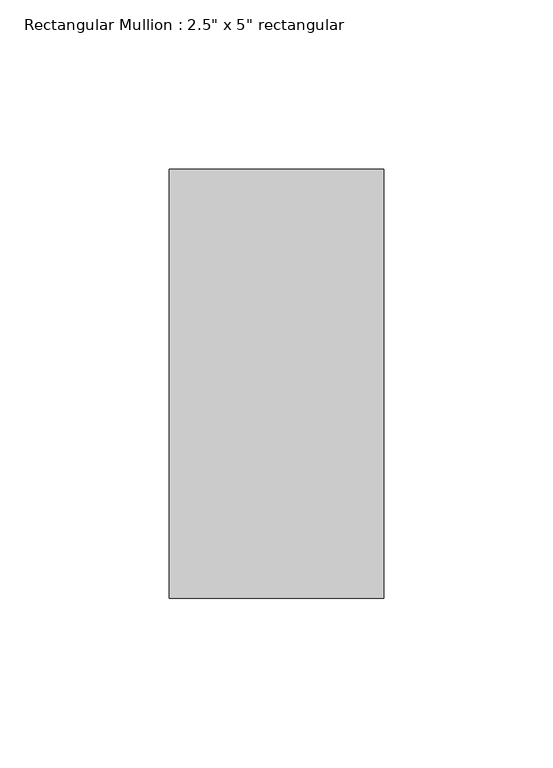
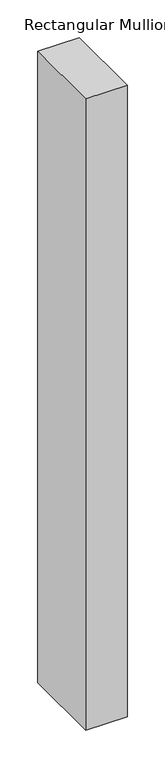
"""IFC4 building model written with IfcOpenShell, lengths in millimetres: member geometry."""

from ifc_helpers import new_model, si_unit, frame, origin, place, context, project, spatial, polyline, outline, extrude, source, transform, mapped, element, save


def member_a1c24a98(model_context):
    return source(origin(), model_context, "Body", "SweptSolid", [
        extrude(outline(polyline([(0.0, 63.5), (0.0, -63.5), (-63.5, -63.5), (-63.5, 63.5), (0.0, 63.5)])), frame((0.0, 0.0, -1022.35), z_axis=(0.0, 0.0, 1.0), x_axis=(1.0, 0.0, 0.0)), (0.0, 0.0, 1.0), 1022.35),
    ])


if __name__ == "__main__":
    model = new_model("IFC4")
    model_context = context("Model", 3, world=origin())
    ifc_project = project(units=[si_unit("LENGTHUNIT", "METRE", prefix="MILLI")], contexts=[model_context])
    site = spatial("IfcSite", under=ifc_project)
    building = spatial("IfcBuilding", under=site)
    placement = place(None, origin())
    member_shape = member_a1c24a98(model_context)
    element("IfcMember", 1, ObjectType="Rectangular Mullion : 2.5\" x 5\" rectangular", at=placement, inside=building, context=model_context, shape_type="MappedRepresentation", body=[
        mapped(member_shape, transform((0.0, 0.0, 0.0), x_axis=(1.0, 0.0, 0.0), y_axis=(0.0, 1.0, 0.0), z_axis=(0.0, 0.0, 1.0))),
    ])
    save(model, "model.ifc")

# Revit data of these elements
# Type "Rectangular Mullion : 2.5\" x 5\" rectangular"
#   built-in parameter 1007304 = 0.416667 (stored number, unit not read)
#   built-in parameter 1007301 = 0.104167 (stored number, unit not read)
#   built-in parameter 1007300 = 0.104167 (stored number, unit not read)
# Element 1 (IfcMember, "Rectangular Mullion : 2.5\" x 5\" rectangular")
#   Materials on its faces: "Aluminum"
# Materials
#   "Aluminum": class "Metal", colour RGB 247 247 247, transparency 0, Description = "Aluminum 6061", Cost = 0
